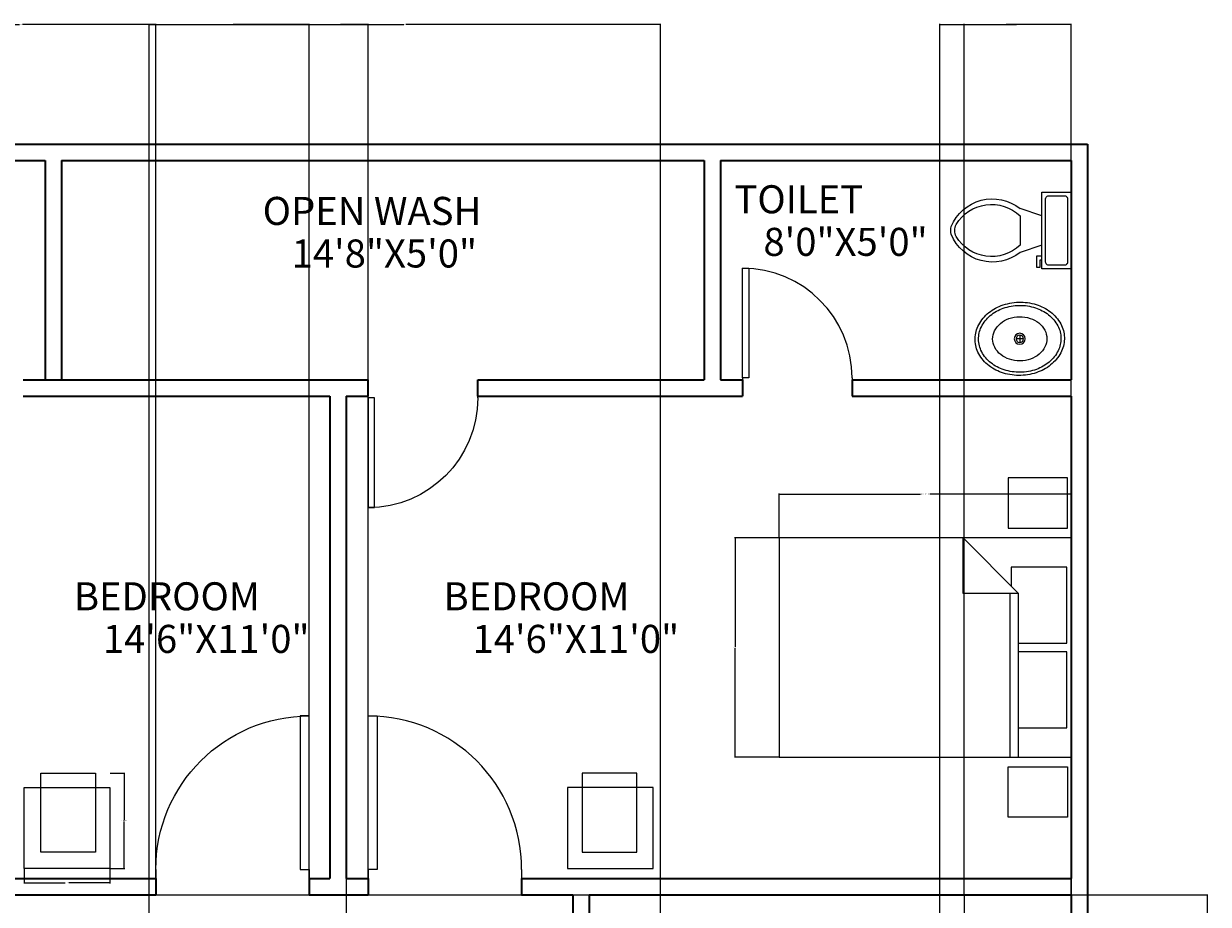
# Model space of a CAD drawing. Units: inches. Extents: x 2337 to 2851, y 1463 to 2183.
# Tile 4 of 4: x 2527 to 2851, y 1942 to 2183. Entities that reach past the tile are written whole.
import ezdxf

# ---------------------------------------------------------------- set-up
doc = ezdxf.new("R2010")
doc.units = ezdxf.units.IN
for name, color, linetype, lineweight in [('A-ANNO-DIMS', 2, 'Continuous', 18), ('A-AREA-IDEN', 7, 'Continuous', 18), ('A-DOOR', 4, 'Continuous', 25), ('A-FLOR-CASE', 8, 'Continuous', 25), ('A-FLOR-FIXT', 9, 'Continuous', 18), ('A-FURN', 8, 'Continuous', 18), ('A-WALL', 7, 'Continuous', 35)]:
    doc.layers.add(name, color=color, linetype=linetype, lineweight=lineweight)
doc.styles.get("Standard").update_dxf_attribs({"font": 'arial.ttf'})
doc.dimstyles.get("Standard").update_dxf_attribs({"dimtxt": 0.18, "dimasz": 0.18, "dimexe": 0.18, "dimexo": 0.0625, "dimgap": 0.09, "dimtad": 0, "dimtih": 1, "dimtoh": 1, "dimdec": 4, "dimzin": 0, "dimdsep": 46, "dimtxsty": 'Standard', "dimcen": 0.09, "dimadec": 0, "dimazin": 0, "dimtfac": 1, "dimtdec": 4, "dimtofl": 0, "dimtmove": 0, "dimatfit": 3, "dimfxl": 1, "dimtolj": 1, "dimtzin": 0, "dimarcsym": 0})

# ---------------------------------------------------------------- blocks, each defined once
blk = doc.blocks.new('*U2')
for p, q in [((0, 0), (0, -5)), ((30, 0), (30, -5))]:
    blk.add_line(p, q)
blk.add_lwpolyline([(0, 0), (0, 30), (1.75, 30), (1.75, 0)], close=True)
blk.add_arc((0, 0), 30, 0, 90)
blk = doc.blocks.new('Toilet - top')
for p, q in [((9.5, -6), (9.5, -2)), ((-10, -8.5), (-8, -8.5)), ((-10, -9.5), (-10, -8.5)), ((-7, -9.5), (-10, -9.5)), ((-8, -8.5), (-8, -8)), ((-7, -8), (-7, -9.5)), ((-4, -8), (-6, -14)), ((4, -8), (6, -14)), ((4, -14), (-4, -14))]:
    blk.add_line(p, q)
blk.add_lwpolyline([(10.5, -8), (10.5, 0), (-10.5, 0), (-10.5, -8)], close=True)
for points in [[(-9.5, -2), (-9.5, -6)], [(8.5, -1), (-8.5, -1)], [(-8.5, -7), (8.5, -7)]]:
    blk.add_lwpolyline(points)
for centre, radius, start, end in [((-8.62, -1.88), 0.884, 81.8699, 188.1301), ((8.62, -1.88), 0.884, 351.8699, 98.1301), ((-8.62, -6.12), 0.884, 171.8699, 278.1301), ((8.62, -6.12), 0.884, 261.8699, 8.1301), ((3.52, -21.58), 12.17, 141.4691, 247.9714), ((4.2, -21.82), 11.33, 136.3677, 238.9468), ((-3.52, -21.58), 12.17, 292.0284, 38.5307), ((-4.2, -21.82), 11.33, 301.053, 43.6321), ((0, -27.88), 4, 245.7318, 294.2682), ((0, -29), 4, 254.8605, 285.1395)]:
    blk.add_arc(centre, radius, start, end)
blk = doc.blocks.new('Sink - Oval top')
for p, q in [((-1, 0), (1, 0)), ((0, 1), (0, -1))]:
    blk.add_line(p, q)
for points in [[(-12.23, 0.39, 0.117634), (-11.46, -3.36, 0.104469), (-8.88, -6.8, 0.090016), (-5.08, -9.07, 0.08192), (-0.32, -10.02, 0.08192), (4.49, -9.38, 0.090016), (8.42, -7.36, 0.104469), (11.22, -4.09, 0.117634), (12.23, -0.39, 0.117634), (11.46, 3.36, 0.104469), (8.88, 6.8, 0.090016), (5.08, 9.07, 0.08192), (0.32, 10.02, 0.08192), (-4.49, 9.38, 0.090016), (-8.42, 7.36, 0.104469), (-11.22, 4.09, 0.117634)], [(-11.29, 0.16, 0.118622), (-10.52, -3.25, 0.104678), (-8.07, -6.36, 0.089562), (-4.54, -8.37, 0.081185), (-0.13, -9.15, 0.081185), (4.3, -8.49, 0.089562), (7.89, -6.58, 0.104678), (10.42, -3.55, 0.118622), (11.29, -0.16, 0.118622), (10.52, 3.25, 0.104678), (8.07, 6.36, 0.089562), (4.54, 8.37, 0.081185), (0.13, 9.15, 0.081185), (-4.3, 8.49, 0.089562), (-7.89, 6.58, 0.104678), (-10.42, 3.55, 0.118622)], [(-7.42, 0.08, 0.118283), (-6.91, -2.17, 0.104607), (-5.29, -4.21, 0.089718), (-2.97, -5.53, 0.081436), (-0.07, -6.04, 0.081436), (2.84, -5.59, 0.089718), (5.2, -4.33, 0.104607), (6.86, -2.32, 0.118283), (7.42, -0.08, 0.118283), (6.91, 2.17, 0.104607), (5.29, 4.21, 0.089718), (2.97, 5.53, 0.081436), (0.07, 6.04, 0.081436), (-2.84, 5.59, 0.089718), (-5.2, 4.33, 0.104607), (-6.86, 2.32, 0.118283)]]:
    blk.add_lwpolyline(points, format="xyb", close=True)
for radius in [1.5, 1]:
    blk.add_circle((0, 0), radius)
blk = doc.blocks.new('Bed - Queen')
for p, q in [((0, -80.00003), (0, 0)), ((0, 0), (59.99999, 0)), ((59.99999, 0), (59.99999, -80.00003)), ((7.99999, -1.2), (28.79998, -1.2)), ((7.99999, -14.4), (7.99999, -1.2)), ((28.79998, -1.2), (28.79998, -14.4)), ((31.19999, -1.2), (51.99999, -1.2)), ((31.19999, -14.4), (31.19999, -1.2)), ((51.99999, -1.2), (51.99999, -16.4)), ((0, -14.4), (44.8, -14.4)), ((59.99999, -29.6), (44.8, -14.4)), ((44.8, -14.4), (44.8, -29.6)), ((44.8, -16.8), (0, -16.8)), ((51.99999, -16.4), (46.79936, -16.4)), ((44.8, -29.6), (59.99999, -29.6)), ((59.99999, -80.00003), (0, -80.00003))]:
    blk.add_line(p, q)
blk = doc.blocks.new('NIGHTSTAND')
blk.add_lwpolyline([(0, 13.73), (16.32, 13.73), (16.32, 0), (0, 0)], close=True)
blk = doc.blocks.new('BEDROOM-CHAIR')
for points in [[(4.51, 26.13), (19.48, 26.13), (19.48, 4.51), (4.51, 4.51)], [(0, 22.16), (23.45, 22.16), (23.45, 0), (0, 0)]]:
    blk.add_lwpolyline(points, close=True)
blk = doc.blocks.new('*D15')
at = {"layer": 'A-ANNO-DIMS', "color": 0, "lineweight": -2, "transparency": 16777216}
for p, q in [((2733.54, 2042.1), (2733.54, 2054.21)), ((2733.72, 2054.03), (2772.23, 2054.03)), ((2813.36, 2054.03), (2774.84, 2054.03)), ((2813.54, 2042.1), (2813.54, 2054.21))]:
    blk.add_line(p, q, dxfattribs=at)
at = {"layer": 'A-ANNO-DIMS', "color": 0, "transparency": 16777216}
for points in [[(2733.72, 2054.06), (2733.72, 2054), (2733.54, 2054.03)], [(2813.36, 2054.06), (2813.36, 2054), (2813.54, 2054.03)]]:
    blk.add_solid(points, dxfattribs=at)
at = {"layer": 'Defpoints', "color": 0, "transparency": 16777216}
for p in [(2813.54, 2054.03), (2733.54, 2042.03), (2813.54, 2042.03)]:
    blk.add_point(p, dxfattribs=at)
at = {"layer": 'A-ANNO-DIMS', "color": 0, "transparency": 16777216, "insert": (2773.54, 2054.03), "char_height": 0.18, "attachment_point": 5}
blk.add_mtext('\\A1;QUEEN BED 80 TYP.', dxfattribs=at)
blk = doc.blocks.new('*D16')
at = {"layer": 'A-ANNO-DIMS', "color": 0, "lineweight": -2, "transparency": 16777216}
for p, q in [((2733.47, 2042.03), (2721.36, 2042.03)), ((2721.54, 2041.85), (2721.54, 2012.22)), ((2721.54, 1982.21), (2721.54, 2011.85)), ((2733.47, 1982.03), (2721.36, 1982.03))]:
    blk.add_line(p, q, dxfattribs=at)
at = {"layer": 'A-ANNO-DIMS', "color": 0, "transparency": 16777216}
for points in [[(2721.51, 2041.85), (2721.57, 2041.85), (2721.54, 2042.03)], [(2721.51, 1982.21), (2721.57, 1982.21), (2721.54, 1982.03)]]:
    blk.add_solid(points, dxfattribs=at)
at = {"layer": 'Defpoints', "color": 0, "transparency": 16777216}
for p in [(2721.54, 2042.03), (2733.54, 2042.03), (2733.54, 1982.03)]:
    blk.add_point(p, dxfattribs=at)
at = {"layer": 'A-ANNO-DIMS', "color": 0, "transparency": 16777216, "insert": (2721.54, 2012.03), "char_height": 0.18, "attachment_point": 5}
blk.add_mtext('\\A1;60 TYP.', dxfattribs=at)
blk = doc.blocks.new('*D17')
at = {"layer": 'A-ANNO-DIMS', "color": 0, "lineweight": -2, "transparency": 16777216}
for p, q in [((2550.36, 1977.7), (2554.39, 1977.7)), ((2554.21, 1977.52), (2554.21, 1964.82)), ((2554.21, 1951.75), (2554.21, 1964.45)), ((2550.36, 1951.57), (2554.39, 1951.57))]:
    blk.add_line(p, q, dxfattribs=at)
at = {"layer": 'A-ANNO-DIMS', "color": 0, "transparency": 16777216}
for points in [[(2554.18, 1977.52), (2554.24, 1977.52), (2554.21, 1977.7)], [(2554.18, 1951.75), (2554.24, 1951.75), (2554.21, 1951.57)]]:
    blk.add_solid(points, dxfattribs=at)
at = {"layer": 'Defpoints', "color": 0, "transparency": 16777216}
for p in [(2550.29, 1977.7), (2554.21, 1977.7), (2550.29, 1951.57)]:
    blk.add_point(p, dxfattribs=at)
at = {"layer": 'A-ANNO-DIMS', "color": 0, "transparency": 16777216, "insert": (2554.21, 1964.63), "char_height": 0.18, "attachment_point": 5}
blk.add_mtext('\\A1;CHAIR 26 TYP.', dxfattribs=at)
blk = doc.blocks.new('*D18')
at = {"layer": 'A-ANNO-DIMS', "color": 0, "lineweight": -2, "transparency": 16777216}
for p, q in [((2526.85, 1951.51), (2526.85, 1947.47)), ((2550.29, 1951.51), (2550.29, 1947.47)), ((2527.03, 1947.65), (2538.04, 1947.65)), ((2550.11, 1947.65), (2539.1, 1947.65))]:
    blk.add_line(p, q, dxfattribs=at)
at = {"layer": 'A-ANNO-DIMS', "color": 0, "transparency": 16777216}
for points in [[(2527.03, 1947.68), (2527.03, 1947.62), (2526.85, 1947.65)], [(2550.11, 1947.68), (2550.11, 1947.62), (2550.29, 1947.65)]]:
    blk.add_solid(points, dxfattribs=at)
at = {"layer": 'Defpoints', "color": 0, "transparency": 16777216}
for p in [(2526.85, 1951.57), (2550.29, 1951.57), (2550.29, 1947.65)]:
    blk.add_point(p, dxfattribs=at)
at = {"layer": 'A-ANNO-DIMS', "color": 0, "transparency": 16777216, "insert": (2538.57, 1947.65), "char_height": 0.18, "attachment_point": 5}
blk.add_mtext('\\A1;23 TYP.', dxfattribs=at)
blk = doc.blocks.new('*D32')
at = {"layer": 'A-ANNO-DIMS', "color": 0, "lineweight": -2, "transparency": 16777216}
for p, q in [((2561.04, 1627.89), (2561.04, 2182.75)), ((2561.22, 2182.57), (2630.76, 2182.57)), ((2700.86, 2182.57), (2631.32, 2182.57)), ((2701.04, 1627.89), (2701.04, 2182.75))]:
    blk.add_line(p, q, dxfattribs=at)
at = {"layer": 'A-ANNO-DIMS', "color": 0, "transparency": 16777216}
for points in [[(2561.22, 2182.6), (2561.22, 2182.54), (2561.04, 2182.57)], [(2700.86, 2182.6), (2700.86, 2182.54), (2701.04, 2182.57)]]:
    blk.add_solid(points, dxfattribs=at)
at = {"layer": 'Defpoints', "color": 0, "transparency": 16777216}
for p in [(2701.04, 2182.57), (2561.04, 1627.83), (2701.04, 1627.83)]:
    blk.add_point(p, dxfattribs=at)
at = {"layer": 'A-ANNO-DIMS', "color": 0, "transparency": 16777216, "insert": (2631.04, 2182.57), "char_height": 0.18, "attachment_point": 5}
blk.add_mtext('\\A1;140', dxfattribs=at)
blk = doc.blocks.new('*D36')
at = {"layer": 'A-ANNO-DIMS', "color": 0, "lineweight": -2, "transparency": 16777216}
for p, q in [((2489.1, 1944.33), (2850.96, 1944.33)), ((2850.78, 1944.15), (2850.78, 1878.51)), ((2850.78, 1812.51), (2850.78, 1878.15)), ((2489.1, 1812.33), (2850.96, 1812.33))]:
    blk.add_line(p, q, dxfattribs=at)
at = {"layer": 'A-ANNO-DIMS', "color": 0, "transparency": 16777216}
for points in [[(2850.75, 1944.15), (2850.81, 1944.15), (2850.78, 1944.33)], [(2850.75, 1812.51), (2850.81, 1812.51), (2850.78, 1812.33)]]:
    blk.add_solid(points, dxfattribs=at)
at = {"layer": 'Defpoints', "color": 0, "transparency": 16777216}
for p in [(2489.04, 1944.33), (2850.78, 1944.33), (2489.04, 1812.33)]:
    blk.add_point(p, dxfattribs=at)
at = {"layer": 'A-ANNO-DIMS', "color": 0, "transparency": 16777216, "insert": (2850.78, 1878.33), "char_height": 0.18, "attachment_point": 5}
blk.add_mtext('\\A1;132', dxfattribs=at)
blk = doc.blocks.new('*D37')
at = {"layer": 'A-ANNO-DIMS', "color": 0, "lineweight": -2, "transparency": 16777216}
for p, q in [((2615.04, 2080.77), (2615.04, 1462.52)), ((2813.54, 2080.77), (2813.54, 1462.52)), ((2615.22, 1462.7), (2713.9, 1462.7)), ((2813.36, 1462.7), (2714.67, 1462.7))]:
    blk.add_line(p, q, dxfattribs=at)
at = {"layer": 'A-ANNO-DIMS', "color": 0, "transparency": 16777216}
for points in [[(2615.22, 1462.73), (2615.22, 1462.67), (2615.04, 1462.7)], [(2813.36, 1462.73), (2813.36, 1462.67), (2813.54, 1462.7)]]:
    blk.add_solid(points, dxfattribs=at)
at = {"layer": 'Defpoints', "color": 0, "transparency": 16777216}
for p in [(2615.04, 2080.83), (2813.54, 2080.83), (2813.54, 1462.7)]:
    blk.add_point(p, dxfattribs=at)
at = {"layer": 'A-ANNO-DIMS', "color": 0, "transparency": 16777216, "insert": (2714.29, 1462.7), "char_height": 0.18, "attachment_point": 5}
blk.add_mtext('\\A1;198.5', dxfattribs=at)
blk = doc.blocks.new('*D40')
at = {"layer": 'A-ANNO-DIMS', "color": 0, "lineweight": -2, "transparency": 16777216}
for p, q in [((2562.88, 1948.89), (2562.88, 2182.75)), ((2563.06, 2182.57), (2583.66, 2182.57)), ((2604.7, 2182.57), (2584.1, 2182.57)), ((2604.88, 1948.89), (2604.88, 2182.75))]:
    blk.add_line(p, q, dxfattribs=at)
at = {"layer": 'A-ANNO-DIMS', "color": 0, "transparency": 16777216}
for points in [[(2563.06, 2182.6), (2563.06, 2182.54), (2562.88, 2182.57)], [(2604.7, 2182.6), (2604.7, 2182.54), (2604.88, 2182.57)]]:
    blk.add_solid(points, dxfattribs=at)
at = {"layer": 'Defpoints', "color": 0, "transparency": 16777216}
for p in [(2604.88, 2182.57), (2562.88, 1948.83), (2604.88, 1948.83)]:
    blk.add_point(p, dxfattribs=at)
at = {"layer": 'A-ANNO-DIMS', "color": 0, "transparency": 16777216, "insert": (2583.88, 2182.57), "char_height": 0.18, "attachment_point": 5}
blk.add_mtext('\\A1;42', dxfattribs=at)
blk = doc.blocks.new('*D42')
at = {"layer": 'A-ANNO-DIMS', "color": 0, "lineweight": -2, "transparency": 16777216}
for p, q in [((2681.6, 1944.33), (2850.96, 1944.33)), ((2850.78, 1944.15), (2850.78, 1921.51)), ((2850.78, 1898.52), (2850.78, 1921.15)), ((2681.6, 1898.34), (2850.96, 1898.34))]:
    blk.add_line(p, q, dxfattribs=at)
at = {"layer": 'A-ANNO-DIMS', "color": 0, "transparency": 16777216}
for points in [[(2850.75, 1944.15), (2850.81, 1944.15), (2850.78, 1944.33)], [(2850.75, 1898.52), (2850.81, 1898.52), (2850.78, 1898.34)]]:
    blk.add_solid(points, dxfattribs=at)
at = {"layer": 'Defpoints', "color": 0, "transparency": 16777216}
for p in [(2681.54, 1944.33), (2850.78, 1944.33), (2681.54, 1898.34)]:
    blk.add_point(p, dxfattribs=at)
at = {"layer": 'A-ANNO-DIMS', "color": 0, "transparency": 16777216, "insert": (2850.78, 1921.33), "char_height": 0.18, "attachment_point": 5}
blk.add_mtext('\\A1;45.99', dxfattribs=at)
blk = doc.blocks.new('*D45')
at = {"layer": 'A-ANNO-DIMS', "color": 0, "lineweight": -2, "transparency": 16777216}
for p, q in [((2777.54, 1699.89), (2777.54, 2182.75)), ((2777.72, 2182.57), (2795.32, 2182.57)), ((2813.36, 2182.57), (2795.76, 2182.57)), ((2813.54, 1699.89), (2813.54, 2182.75))]:
    blk.add_line(p, q, dxfattribs=at)
at = {"layer": 'A-ANNO-DIMS', "color": 0, "transparency": 16777216}
for points in [[(2777.72, 2182.6), (2777.72, 2182.54), (2777.54, 2182.57)], [(2813.36, 2182.6), (2813.36, 2182.54), (2813.54, 2182.57)]]:
    blk.add_solid(points, dxfattribs=at)
at = {"layer": 'Defpoints', "color": 0, "transparency": 16777216}
for p in [(2813.54, 2182.57), (2777.54, 1699.83), (2813.54, 1699.83)]:
    blk.add_point(p, dxfattribs=at)
at = {"layer": 'A-ANNO-DIMS', "color": 0, "transparency": 16777216, "insert": (2795.54, 2182.57), "char_height": 0.18, "attachment_point": 5}
blk.add_mtext('\\A1;36', dxfattribs=at)
blk = doc.blocks.new('*D47')
at = {"layer": 'A-ANNO-DIMS', "color": 0, "lineweight": -2, "transparency": 16777216}
for p, q in [((2784.24, 1944.39), (2784.24, 2182.75)), ((2784.42, 2182.57), (2798.56, 2182.57)), ((2813.36, 2182.57), (2799.21, 2182.57)), ((2813.54, 1944.39), (2813.54, 2182.75))]:
    blk.add_line(p, q, dxfattribs=at)
at = {"layer": 'A-ANNO-DIMS', "color": 0, "transparency": 16777216}
for points in [[(2784.42, 2182.6), (2784.42, 2182.54), (2784.24, 2182.57)], [(2813.36, 2182.6), (2813.36, 2182.54), (2813.54, 2182.57)]]:
    blk.add_solid(points, dxfattribs=at)
at = {"layer": 'Defpoints', "color": 0, "transparency": 16777216}
for p in [(2813.54, 2182.57), (2784.24, 1944.33), (2813.54, 1944.33)]:
    blk.add_point(p, dxfattribs=at)
at = {"layer": 'A-ANNO-DIMS', "color": 0, "transparency": 16777216, "insert": (2798.89, 2182.57), "char_height": 0.18, "attachment_point": 5}
blk.add_mtext('\\A1;29.3', dxfattribs=at)
blk = doc.blocks.new('*D57')
at = {"layer": 'A-ANNO-DIMS', "color": 0, "lineweight": -2, "transparency": 16777216}
for p, q in [((2489.04, 1944.39), (2489.04, 2182.75)), ((2489.22, 2182.57), (2525.57, 2182.57)), ((2562.7, 2182.57), (2526.35, 2182.57)), ((2562.88, 1944.39), (2562.88, 2182.75))]:
    blk.add_line(p, q, dxfattribs=at)
at = {"layer": 'A-ANNO-DIMS', "color": 0, "transparency": 16777216}
for points in [[(2489.22, 2182.6), (2489.22, 2182.54), (2489.04, 2182.57)], [(2562.7, 2182.6), (2562.7, 2182.54), (2562.88, 2182.57)]]:
    blk.add_solid(points, dxfattribs=at)
at = {"layer": 'Defpoints', "color": 0, "transparency": 16777216}
for p in [(2562.88, 2182.57), (2489.04, 1944.33), (2562.88, 1944.33)]:
    blk.add_point(p, dxfattribs=at)
at = {"layer": 'A-ANNO-DIMS', "color": 0, "transparency": 16777216, "insert": (2525.96, 2182.57), "char_height": 0.18, "attachment_point": 5}
blk.add_mtext('\\A1;73.84', dxfattribs=at)
blk = doc.blocks.new('*D58')
at = {"layer": 'A-ANNO-DIMS', "color": 0, "lineweight": -2, "transparency": 16777216}
for p, q in [((2604.88, 1944.39), (2604.88, 2182.75)), ((2605.06, 2182.57), (2612.5, 2182.57)), ((2620.86, 2182.57), (2613.41, 2182.57)), ((2621.04, 1944.39), (2621.04, 2182.75))]:
    blk.add_line(p, q, dxfattribs=at)
at = {"layer": 'A-ANNO-DIMS', "color": 0, "transparency": 16777216}
for points in [[(2605.06, 2182.6), (2605.06, 2182.54), (2604.88, 2182.57)], [(2620.86, 2182.6), (2620.86, 2182.54), (2621.04, 2182.57)]]:
    blk.add_solid(points, dxfattribs=at)
at = {"layer": 'Defpoints', "color": 0, "transparency": 16777216}
for p in [(2621.04, 2182.57), (2604.88, 1944.33), (2621.04, 1944.33)]:
    blk.add_point(p, dxfattribs=at)
at = {"layer": 'A-ANNO-DIMS', "color": 0, "transparency": 16777216, "insert": (2612.96, 2182.57), "char_height": 0.18, "attachment_point": 5}
blk.add_mtext('\\A1;16.158', dxfattribs=at)

msp = doc.modelspace()

# ---------------------------------------------------------------- linework, layer by layer
at = {"layer": 'A-FLOR-CASE'}
msp.add_line((2784.2391, 1944.328), (2784.2391, 1845.4107), dxfattribs=at)
at = {"layer": 'A-WALL'}
for p, q in [((2432.0375, 2149.828), (2818.0375, 2149.828)), ((2432.0375, 2149.828), (2818.0375, 2149.828)), ((2818.0375, 2149.828), (2818.0375, 1557.328)), ((2436.5375, 2145.328), (2532.5375, 2145.328)), ((2532.5375, 2145.328), (2532.5375, 2085.328)), ((2537.0375, 2145.328), (2537.0375, 2085.328)), ((2537.0375, 2145.328), (2713.0375, 2145.328)), ((2713.0375, 2145.328), (2713.0375, 2085.328)), ((2717.5375, 2145.328), (2717.5375, 2085.328)), ((2717.5375, 2145.328), (2813.5375, 2145.328)), ((2813.5375, 2145.328), (2813.5375, 2085.328)), ((2526.5375, 2085.328), (2621.0375, 2085.328)), ((2621.0375, 2080.828), (2621.0375, 2085.328)), ((2651.0375, 2080.828), (2651.0375, 2085.328)), ((2651.0375, 2085.328), (2713.0375, 2085.328)), ((2717.5375, 2085.328), (2723.5375, 2085.328)), ((2723.5375, 2085.328), (2723.5375, 2080.828)), ((2753.5375, 2085.328), (2753.5375, 2080.828)), ((2753.5375, 2085.328), (2813.5375, 2085.328)), ((2526.5375, 2080.828), (2610.5375, 2080.828)), ((2610.5375, 2080.828), (2610.5375, 1948.828)), ((2615.0375, 2080.828), (2615.0375, 1948.828)), ((2615.0375, 2080.828), (2621.0375, 2080.828)), ((2651.0375, 2080.828), (2723.5375, 2080.828)), ((2753.5375, 2080.828), (2813.5375, 2080.828)), ((2813.5375, 2080.828), (2813.5375, 1948.828)), ((2436.5375, 1948.828), (2562.8796, 1948.828)), ((2562.8796, 1948.828), (2562.8796, 1944.328)), ((2604.8796, 1948.828), (2604.8796, 1944.328)), ((2604.8796, 1948.828), (2610.5375, 1948.828)), ((2615.0375, 1948.828), (2621.0375, 1948.828)), ((2621.0375, 1948.828), (2621.0375, 1944.328)), ((2663.0375, 1948.828), (2663.0375, 1944.328)), ((2663.0375, 1948.828), (2813.5375, 1948.828)), ((2489.0375, 1944.328), (2562.8796, 1944.328)), ((2604.8796, 1944.328), (2621.0375, 1944.328)), ((2663.0375, 1944.328), (2677.0375, 1944.328)), ((2677.0375, 1944.328), (2677.0375, 1898.3363)), ((2681.5375, 1944.328), (2681.5375, 1898.3363)), ((2681.5375, 1944.328), (2813.5375, 1944.328)), ((2813.5375, 1944.328), (2813.5375, 1812.328))]:
    msp.add_line(p, q, dxfattribs=at)

# ---------------------------------------------------------------- block references
at = {"layer": 'A-DOOR'}
msp.add_blockref('*U2', (2723.5375, 2085.828), dxfattribs=at)
at = {"layer": 'A-DOOR', "xscale": -1, "rotation": 180}
msp.add_blockref('*U2', (2621.0375, 2080.328), dxfattribs=at)
at = {"layer": 'A-DOOR', "yscale": 1.399999999999999, "zscale": 1.399999999999999}
for p, xscale in [((2604.8796, 1951.328), -1.399999999999999), ((2621.0375, 1951.328), 1.399999999999999)]:
    msp.add_blockref('*U2', p, dxfattribs=dict(at, xscale=xscale))
at = {"layer": 'A-FLOR-FIXT', "xscale": -1, "rotation": 270}
msp.add_blockref('Toilet - top', (2813.5375, 2126.1668), dxfattribs=at)
at = {"layer": 'A-FLOR-FIXT', "xscale": -1}
msp.add_blockref('Sink - Oval top', (2799.4515, 2096.5253), dxfattribs=at)
at = {"layer": 'A-FURN', "extrusion": (0, 0, -1), "zscale": -1}
for name, p in [('NIGHTSTAND', (-2812.5689, 2044.705)), ('BEDROOM-CHAIR', (-2699.068, 1951.569))]:
    msp.add_blockref(name, p, dxfattribs=at)
at = {"layer": 'A-FURN', "xscale": -1, "rotation": 270}
msp.add_blockref('Bed - Queen', (2813.5375, 1982.0338), dxfattribs=at)
at = {"layer": 'A-FURN', "rotation": 180}
msp.add_blockref('NIGHTSTAND', (2812.5689, 1979.3626), dxfattribs=at)
at = {"layer": 'A-FURN'}
msp.add_blockref('BEDROOM-CHAIR', (2526.849, 1951.569), dxfattribs=at)

# ---------------------------------------------------------------- texts
at = {"layer": 'A-AREA-IDEN'}
for s, height, p in [('TOILET', 7.67227, (2721.3317, 2130.8688)), ('OPEN WASH', 7.67227, (2592.1368, 2127.6823)), ('8\'0"X5\'0"', 7.67227, (2729.2599, 2119.2171)), ('14\'8"X5\'0"', 7.67227, (2600.065, 2116.0306)), ('BEDROOM', 7.67227, (2540.4581, 2022.2217)), ('BEDROOM', 7.67227, (2641.6728, 2022.2217)), ('14\'6"X11\'0"', 7.672274, (2548.3863, 2010.5699)), ('14\'6"X11\'0"', 7.672274, (2649.601, 2010.5699))]:
    msp.add_text(s, height=height, dxfattribs=at).set_placement(p)

# ---------------------------------------------------------------- dimensions: what is measured, and where the dimension line sits
at = {"layer": 'A-ANNO-DIMS'}
for base, p1, p2, override, picture, middle in [((2562.8796, 2182.568), (2489.0375, 1944.328), (2562.8796, 1944.328), {"dimdec": 2, "dimlfac": 1, "dimrnd": 0, "dimzin": 0, "dimdsep": 46, "dimlunit": 2}, '*D57', (2525.9585, 2182.568)), ((2701.0375, 2182.568), (2561.0375, 1627.828), (2701.0375, 1627.828), {"dimdec": 0, "dimlfac": 1, "dimrnd": 0, "dimzin": 0, "dimdsep": 46, "dimlunit": 2}, '*D32', (2631.0375, 2182.568)), ((2604.8796, 2182.568), (2562.8796, 1948.828), (2604.8796, 1948.828), {"dimdec": 0, "dimlfac": 1, "dimrnd": 0, "dimzin": 0, "dimdsep": 46, "dimlunit": 2}, '*D40', (2583.8796, 2182.568)), ((2621.0375, 2182.568), (2604.8796, 1944.328), (2621.0375, 1944.328), {"dimdec": 3, "dimlfac": 1, "dimrnd": 0, "dimzin": 0, "dimdsep": 46, "dimlunit": 2}, '*D58', (2612.9585, 2182.568)), ((2813.5375, 2182.568), (2777.5375, 1699.828), (2813.5375, 1699.828), {"dimdec": 0, "dimlfac": 1, "dimrnd": 0, "dimzin": 0, "dimdsep": 46, "dimlunit": 2}, '*D45', (2795.5375, 2182.568)), ((2813.5375, 2182.568), (2784.2391, 1944.328), (2813.5375, 1944.328), {"dimdec": 1, "dimlfac": 1, "dimrnd": 0, "dimzin": 0, "dimdsep": 46, "dimlunit": 2}, '*D47', (2798.8883, 2182.568)), ((2813.5375, 1462.7036), (2615.0375, 2080.828), (2813.5375, 2080.828), {"dimdec": 1, "dimlfac": 1, "dimrnd": 0, "dimzin": 0, "dimdsep": 46, "dimlunit": 2}, '*D37', (2714.2875, 1462.7036))]:
    dim = msp.add_linear_dim(base=base, p1=p1, p2=p2, dimstyle='Standard', override=override, dxfattribs=at)
    dim.commit()
    dim.dimension.update_dxf_attribs({"geometry": picture, "text_midpoint": middle})
for base, p1, p2, text, picture, middle in [((2813.5375, 2054.0338), (2733.5374, 2042.0338), (2813.5375, 2042.0338), 'QUEEN BED <> TYP.', '*D15', (2773.5374, 2054.0338)), ((2550.2947, 1947.6499), (2526.8494, 1951.5689), (2550.2947, 1951.5689), '<> TYP.', '*D18', (2538.5721, 1947.6499))]:
    dim = msp.add_linear_dim(base=base, p1=p1, p2=p2, text=text, dimstyle='Standard', override={"dimdec": 0, "dimlfac": 1, "dimrnd": 0, "dimzin": 0, "dimdsep": 46, "dimlunit": 2}, dxfattribs=at)
    dim.commit()
    dim.dimension.update_dxf_attribs({"geometry": picture, "text_midpoint": middle})
for base, p1, p2, text, picture, middle in [((2721.5374, 2042.0338), (2733.5374, 1982.0338), (2733.5374, 2042.0338), '<> TYP.', '*D16', (2721.5374, 2012.0338)), ((2554.2137, 1977.6954), (2550.2947, 1951.5689), (2550.2947, 1977.6954), 'CHAIR <> TYP.', '*D17', (2554.2137, 1964.6321))]:
    dim = msp.add_linear_dim(base=base, p1=p1, p2=p2, angle=90, text=text, dimstyle='Standard', override={"dimdec": 0, "dimlfac": 1, "dimrnd": 0, "dimzin": 0, "dimdsep": 46, "dimlunit": 2}, dxfattribs=at)
    dim.commit()
    dim.dimension.update_dxf_attribs({"geometry": picture, "text_midpoint": middle})
for p1, p2, override, picture, middle in [((2489.0375, 1812.328), (2489.0375, 1944.328), {"dimdec": 0, "dimlfac": 1, "dimrnd": 0, "dimzin": 0, "dimdsep": 46, "dimlunit": 2}, '*D36', (2850.7775, 1878.328)), ((2681.5375, 1898.3363), (2681.5375, 1944.328), {"dimdec": 2, "dimlfac": 1, "dimrnd": 0, "dimzin": 0, "dimdsep": 46, "dimlunit": 2}, '*D42', (2850.7775, 1921.3321))]:
    dim = msp.add_linear_dim(base=(2850.7775, 1944.328), p1=p1, p2=p2, angle=90, dimstyle='Standard', override=override, dxfattribs=at)
    dim.commit()
    dim.dimension.update_dxf_attribs({"geometry": picture, "text_midpoint": middle})

doc.saveas('drawing.dxf')
